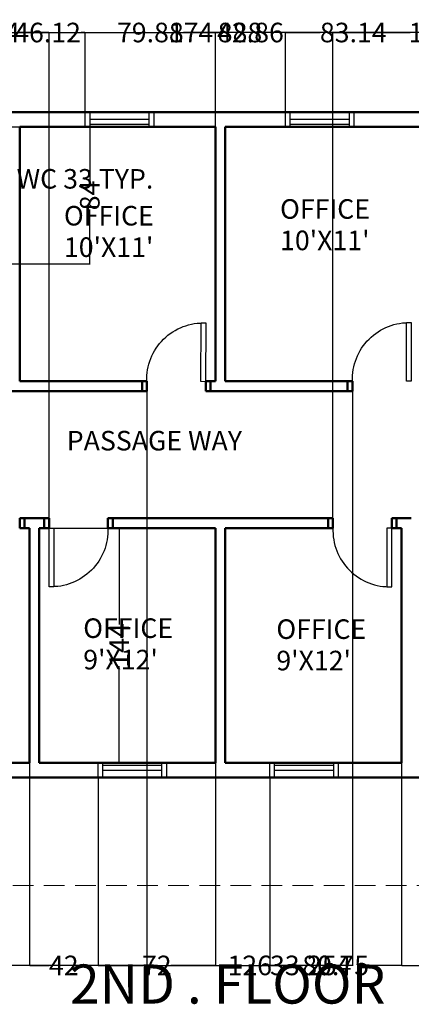
# Model space of a CAD drawing. Units: inches. Extents: x 128 to 1267, y -109 to 1208.
# Tile 7 of 8: x 546 to 786, y 592 to 1196. Entities that reach past the tile are written whole.
import ezdxf

# ---------------------------------------------------------------- set-up
doc = ezdxf.new("R2010")
doc.units = ezdxf.units.IN
doc.header["$MEASUREMENT"] = 0
doc.linetypes.add('DASHED', pattern=[19.05, 12.7, -6.35])
for name, color, linetype, lineweight in [('A-ANNO-DIMS', 2, 'Continuous', 18), ('A-ANNO-TEXT', 7, 'Continuous', 35), ('A-AREA-IDEN', 3, 'Continuous', 25), ('A-DOOR', 4, 'Continuous', 25), ('A-GLAZ', 3, 'Continuous', 25), ('A-ROOF-OVHD', 9, 'DASHED', 18), ('A-WALL', 7, 'Continuous', 50)]:
    doc.layers.add(name, color=color, linetype=linetype, lineweight=lineweight)
doc.styles.get("Standard").update_dxf_attribs({"font": 'arial.ttf'})
doc.dimstyles.get("Standard").update_dxf_attribs({"dimtxt": 12, "dimasz": 0.18, "dimexe": 0.18, "dimexo": 0.0625, "dimgap": 0.09, "dimtad": 0, "dimdec": 1, "dimzin": 0, "dimdsep": 46, "dimlunit": 3, "dimtxsty": 'Standard', "dimcen": 0.09, "dimadec": 0, "dimazin": 0, "dimtfac": 1, "dimtdec": 1, "dimtofl": 0, "dimtmove": 0, "dimatfit": 3, "dimfxl": 1, "dimtolj": 1, "dimtzin": 0, "dimarcsym": 0})

# ---------------------------------------------------------------- blocks, each defined once
blk = doc.blocks.new('DOOR-900')
blk.add_lwpolyline([(460.06, 187.64), (457.06, 187.64), (457.06, 151.64), (460.06, 151.64)], close=True)
blk.add_arc((458.56, 186.14), 34.53, 177.51045, 272.48955)
blk = doc.blocks.new('WIN-900')
for p, q in [((1102.06, 345.56), (1111.06, 345.56)), ((1102.06, 342.56), (1111.06, 342.56)), ((1103.56, 306.56), (1103.56, 342.56)), ((1106.56, 306.56), (1106.56, 342.56)), ((1111.06, 306.56), (1102.06, 306.56)), ((1111.06, 303.56), (1102.06, 303.56))]:
    blk.add_line(p, q)
blk = doc.blocks.new('*D16')
at = {"layer": 'A-ANNO-DIMS', "color": 0, "lineweight": -2, "transparency": 16777216}
for p, q in [((507.08, 1103.32), (507.08, 1098.25)), ((540.13, 1103.32), (540.13, 1098.25)), ((507.26, 1098.43), (539.95, 1098.43)), ((540.13, 1098.43), (540.31, 1098.43))]:
    blk.add_line(p, q, dxfattribs=at)
at = {"layer": 'A-ANNO-DIMS', "color": 0, "transparency": 16777216}
for points in [[(507.26, 1098.46), (507.26, 1098.4), (507.08, 1098.43)], [(539.95, 1098.46), (539.95, 1098.4), (540.13, 1098.43)]]:
    blk.add_solid(points, dxfattribs=at)
at = {"layer": 'Defpoints', "color": 0, "transparency": 16777216}
for p in [(507.08, 1103.38), (540.13, 1103.38), (540.13, 1098.43)]:
    blk.add_point(p, dxfattribs=at)
at = {"layer": 'A-ANNO-DIMS', "color": 0, "transparency": 16777216, "insert": (586.14, 1098.43), "char_height": 12, "attachment_point": 5}
blk.add_mtext('\\A1;WC 33 TYP.', dxfattribs=at)
blk = doc.blocks.new('*D93')
at = {"layer": 'A-ANNO-DIMS', "color": 0, "lineweight": -2, "transparency": 16777216}
for p, q in [((237.13, 664.93), (237.13, 1188.36)), ((237.31, 1188.18), (667.76, 1188.18)), ((1124.95, 1188.18), (694.49, 1188.18)), ((1125.13, 664.93), (1125.13, 1188.36))]:
    blk.add_line(p, q, dxfattribs=at)
at = {"layer": 'A-ANNO-DIMS', "color": 0, "transparency": 16777216}
for points in [[(237.31, 1188.21), (237.31, 1188.15), (237.13, 1188.18)], [(1124.95, 1188.21), (1124.95, 1188.15), (1125.13, 1188.18)]]:
    blk.add_solid(points, dxfattribs=at)
at = {"layer": 'Defpoints', "color": 0, "transparency": 16777216}
for p in [(1125.13, 1188.18), (237.13, 664.87), (1125.13, 664.87)]:
    blk.add_point(p, dxfattribs=at)
at = {"layer": 'A-ANNO-DIMS', "color": 0, "transparency": 16777216, "insert": (681.13, 1188.18), "char_height": 12, "attachment_point": 5}
blk.add_mtext('\\A1;888', dxfattribs=at)
blk = doc.blocks.new('*D103')
at = {"layer": 'A-ANNO-DIMS', "color": 0, "lineweight": -2, "transparency": 16777216}
for p, q in [((540.13, 1130.29), (540.13, 1188.36)), ((540.31, 1188.18), (542.67, 1188.18)), ((586.06, 1188.18), (583.7, 1188.18)), ((586.24, 1139.29), (586.24, 1188.36))]:
    blk.add_line(p, q, dxfattribs=at)
at = {"layer": 'A-ANNO-DIMS', "color": 0, "transparency": 16777216}
for points in [[(540.31, 1188.21), (540.31, 1188.15), (540.13, 1188.18)], [(586.06, 1188.21), (586.06, 1188.15), (586.24, 1188.18)]]:
    blk.add_solid(points, dxfattribs=at)
at = {"layer": 'Defpoints', "color": 0, "transparency": 16777216}
for p in [(586.24, 1188.18), (586.24, 1139.23), (540.13, 1130.23)]:
    blk.add_point(p, dxfattribs=at)
at = {"layer": 'A-ANNO-DIMS', "color": 0, "transparency": 16777216, "insert": (563.19, 1188.18), "char_height": 12, "attachment_point": 5}
blk.add_mtext('\\A1;46.12', dxfattribs=at)
blk = doc.blocks.new('*D104')
at = {"layer": 'A-ANNO-DIMS', "color": 0, "lineweight": -2, "transparency": 16777216}
for p, q in [((586.24, 1139.29), (586.24, 1188.36)), ((586.42, 1188.18), (605.89, 1188.18)), ((665.95, 1188.18), (646.49, 1188.18)), ((666.13, 1130.29), (666.13, 1188.36))]:
    blk.add_line(p, q, dxfattribs=at)
at = {"layer": 'A-ANNO-DIMS', "color": 0, "transparency": 16777216}
for points in [[(586.42, 1188.21), (586.42, 1188.15), (586.24, 1188.18)], [(665.95, 1188.21), (665.95, 1188.15), (666.13, 1188.18)]]:
    blk.add_solid(points, dxfattribs=at)
at = {"layer": 'Defpoints', "color": 0, "transparency": 16777216}
for p in [(666.13, 1188.18), (586.24, 1139.23), (666.13, 1130.23)]:
    blk.add_point(p, dxfattribs=at)
at = {"layer": 'A-ANNO-DIMS', "color": 0, "transparency": 16777216, "insert": (626.19, 1188.18), "char_height": 12, "attachment_point": 5}
blk.add_mtext('\\A1;79.88', dxfattribs=at)
blk = doc.blocks.new('*D105')
at = {"layer": 'A-ANNO-DIMS', "color": 0, "lineweight": -2, "transparency": 16777216}
for p, q in [((666.13, 1130.29), (666.13, 1188.36)), ((666.31, 1188.18), (666.98, 1188.18)), ((708.81, 1188.18), (708.13, 1188.18)), ((708.99, 1139.29), (708.99, 1188.36))]:
    blk.add_line(p, q, dxfattribs=at)
at = {"layer": 'A-ANNO-DIMS', "color": 0, "transparency": 16777216}
for points in [[(666.31, 1188.21), (666.31, 1188.15), (666.13, 1188.18)], [(708.81, 1188.21), (708.81, 1188.15), (708.99, 1188.18)]]:
    blk.add_solid(points, dxfattribs=at)
at = {"layer": 'Defpoints', "color": 0, "transparency": 16777216}
for p in [(708.99, 1188.18), (708.99, 1139.23), (666.13, 1130.23)]:
    blk.add_point(p, dxfattribs=at)
at = {"layer": 'A-ANNO-DIMS', "color": 0, "transparency": 16777216, "insert": (687.56, 1188.18), "char_height": 12, "attachment_point": 5}
blk.add_mtext('\\A1;42.86', dxfattribs=at)
blk = doc.blocks.new('*D106')
at = {"layer": 'A-ANNO-DIMS', "color": 0, "lineweight": -2, "transparency": 16777216}
for p, q in [((708.99, 1139.29), (708.99, 1188.36)), ((709.17, 1188.18), (730.24, 1188.18)), ((791.95, 1188.18), (770.88, 1188.18)), ((792.13, 1130.29), (792.13, 1188.36))]:
    blk.add_line(p, q, dxfattribs=at)
at = {"layer": 'A-ANNO-DIMS', "color": 0, "transparency": 16777216}
for points in [[(709.17, 1188.21), (709.17, 1188.15), (708.99, 1188.18)], [(791.95, 1188.21), (791.95, 1188.15), (792.13, 1188.18)]]:
    blk.add_solid(points, dxfattribs=at)
at = {"layer": 'Defpoints', "color": 0, "transparency": 16777216}
for p in [(792.13, 1188.18), (708.99, 1139.23), (792.13, 1130.23)]:
    blk.add_point(p, dxfattribs=at)
at = {"layer": 'A-ANNO-DIMS', "color": 0, "transparency": 16777216, "insert": (750.56, 1188.18), "char_height": 12, "attachment_point": 5}
blk.add_mtext('\\A1;83.14', dxfattribs=at)
blk = doc.blocks.new('*D115')
at = {"layer": 'A-ANNO-DIMS', "color": 0, "lineweight": -2, "transparency": 16777216}
for p, q in [((552.13, 740.16), (552.13, 615.74)), ((455.08, 731.16), (455.08, 615.74)), ((455.26, 615.92), (483.22, 615.92)), ((551.95, 615.92), (523.98, 615.92))]:
    blk.add_line(p, q, dxfattribs=at)
at = {"layer": 'A-ANNO-DIMS', "color": 0, "transparency": 16777216}
for points in [[(455.26, 615.95), (455.26, 615.89), (455.08, 615.92)], [(551.95, 615.95), (551.95, 615.89), (552.13, 615.92)]]:
    blk.add_solid(points, dxfattribs=at)
at = {"layer": 'Defpoints', "color": 0, "transparency": 16777216}
for p in [(552.13, 740.23), (455.08, 731.23), (552.13, 615.92)]:
    blk.add_point(p, dxfattribs=at)
at = {"layer": 'A-ANNO-DIMS', "color": 0, "transparency": 16777216, "insert": (503.6, 615.92), "char_height": 12, "attachment_point": 5}
blk.add_mtext('\\A1;97.05', dxfattribs=at)
blk = doc.blocks.new('*D116')
at = {"layer": 'A-ANNO-DIMS', "color": 0, "lineweight": -2, "transparency": 16777216}
for p, q in [((552.13, 740.16), (552.13, 615.74)), ((594.13, 731.16), (594.13, 615.74)), ((552.31, 615.92), (564.26, 615.92)), ((593.95, 615.92), (581.99, 615.92))]:
    blk.add_line(p, q, dxfattribs=at)
at = {"layer": 'A-ANNO-DIMS', "color": 0, "transparency": 16777216}
for points in [[(552.31, 615.95), (552.31, 615.89), (552.13, 615.92)], [(593.95, 615.95), (593.95, 615.89), (594.13, 615.92)]]:
    blk.add_solid(points, dxfattribs=at)
at = {"layer": 'Defpoints', "color": 0, "transparency": 16777216}
for p in [(552.13, 740.23), (594.13, 731.23), (594.13, 615.92)]:
    blk.add_point(p, dxfattribs=at)
at = {"layer": 'A-ANNO-DIMS', "color": 0, "transparency": 16777216, "insert": (573.13, 615.92), "char_height": 12, "attachment_point": 5}
blk.add_mtext('\\A1;42', dxfattribs=at)
blk = doc.blocks.new('*D117')
at = {"layer": 'A-ANNO-DIMS', "color": 0, "lineweight": -2, "transparency": 16777216}
for p, q in [((666.13, 740.16), (666.13, 615.74)), ((594.13, 731.16), (594.13, 615.74)), ((594.31, 615.92), (621.55, 615.92)), ((665.95, 615.92), (638.7, 615.92))]:
    blk.add_line(p, q, dxfattribs=at)
at = {"layer": 'A-ANNO-DIMS', "color": 0, "transparency": 16777216}
for points in [[(594.31, 615.95), (594.31, 615.89), (594.13, 615.92)], [(665.95, 615.95), (665.95, 615.89), (666.13, 615.92)]]:
    blk.add_solid(points, dxfattribs=at)
at = {"layer": 'Defpoints', "color": 0, "transparency": 16777216}
for p in [(666.13, 740.23), (594.13, 731.23), (666.13, 615.92)]:
    blk.add_point(p, dxfattribs=at)
at = {"layer": 'A-ANNO-DIMS', "color": 0, "transparency": 16777216, "insert": (630.13, 615.92), "char_height": 12, "attachment_point": 5}
blk.add_mtext('\\A1;72', dxfattribs=at)
blk = doc.blocks.new('*D118')
at = {"layer": 'A-ANNO-DIMS', "color": 0, "lineweight": -2, "transparency": 16777216}
for p, q in [((666.13, 740.16), (666.13, 615.74)), ((699.38, 731.16), (699.38, 615.74)), ((666.31, 615.92), (699.2, 615.92)), ((699.38, 615.92), (699.56, 615.92))]:
    blk.add_line(p, q, dxfattribs=at)
at = {"layer": 'A-ANNO-DIMS', "color": 0, "transparency": 16777216}
for points in [[(666.31, 615.95), (666.31, 615.89), (666.13, 615.92)], [(699.2, 615.95), (699.2, 615.89), (699.38, 615.92)]]:
    blk.add_solid(points, dxfattribs=at)
at = {"layer": 'Defpoints', "color": 0, "transparency": 16777216}
for p in [(666.13, 740.23), (699.38, 731.23), (699.38, 615.92)]:
    blk.add_point(p, dxfattribs=at)
at = {"layer": 'A-ANNO-DIMS', "color": 0, "transparency": 16777216, "insert": (724.53, 615.92), "char_height": 12, "attachment_point": 5}
blk.add_mtext('\\A1;33.254', dxfattribs=at)
blk = doc.blocks.new('*D119')
at = {"layer": 'A-ANNO-DIMS', "color": 0, "lineweight": -2, "transparency": 16777216}
for p, q in [((780.13, 740.16), (780.13, 615.74)), ((699.38, 731.16), (699.38, 615.74)), ((699.56, 615.92), (719.36, 615.92)), ((779.95, 615.92), (760.14, 615.92))]:
    blk.add_line(p, q, dxfattribs=at)
at = {"layer": 'A-ANNO-DIMS', "color": 0, "transparency": 16777216}
for points in [[(699.56, 615.95), (699.56, 615.89), (699.38, 615.92)], [(779.95, 615.95), (779.95, 615.89), (780.13, 615.92)]]:
    blk.add_solid(points, dxfattribs=at)
at = {"layer": 'Defpoints', "color": 0, "transparency": 16777216}
for p in [(780.13, 740.23), (699.38, 731.23), (780.13, 615.92)]:
    blk.add_point(p, dxfattribs=at)
at = {"layer": 'A-ANNO-DIMS', "color": 0, "transparency": 16777216, "insert": (739.75, 615.92), "char_height": 12, "attachment_point": 5}
blk.add_mtext('\\A1;80.75', dxfattribs=at)
blk = doc.blocks.new('*D120')
at = {"layer": 'A-ANNO-DIMS', "color": 0, "lineweight": -2, "transparency": 16777216}
for p, q in [((780.13, 740.16), (780.13, 615.74)), ((802.84, 731.16), (802.84, 615.74)), ((780.31, 615.92), (802.66, 615.92)), ((802.84, 615.92), (803.02, 615.92))]:
    blk.add_line(p, q, dxfattribs=at)
at = {"layer": 'A-ANNO-DIMS', "color": 0, "transparency": 16777216}
for points in [[(780.31, 615.95), (780.31, 615.89), (780.13, 615.92)], [(802.66, 615.95), (802.66, 615.89), (802.84, 615.92)]]:
    blk.add_solid(points, dxfattribs=at)
at = {"layer": 'Defpoints', "color": 0, "transparency": 16777216}
for p in [(780.13, 740.23), (802.84, 731.23), (802.84, 615.92)]:
    blk.add_point(p, dxfattribs=at)
at = {"layer": 'A-ANNO-DIMS', "color": 0, "transparency": 16777216, "insert": (828.1, 615.92), "char_height": 12, "attachment_point": 5}
blk.add_mtext('\\A1;22.714', dxfattribs=at)
blk = doc.blocks.new('*D135')
at = {"layer": 'A-ANNO-DIMS', "color": 0, "lineweight": -2, "transparency": 16777216}
for p, q in [((540.19, 1130.23), (589.26, 1130.23)), ((589.08, 1130.05), (589.08, 1096.89)), ((589.08, 1046.41), (589.08, 1079.56)), ((540.19, 1046.23), (589.26, 1046.23))]:
    blk.add_line(p, q, dxfattribs=at)
at = {"layer": 'A-ANNO-DIMS', "color": 0, "transparency": 16777216}
for points in [[(589.05, 1130.05), (589.11, 1130.05), (589.08, 1130.23)], [(589.05, 1046.41), (589.11, 1046.41), (589.08, 1046.23)]]:
    blk.add_solid(points, dxfattribs=at)
at = {"layer": 'Defpoints', "color": 0, "transparency": 16777216}
for p in [(540.13, 1130.23), (540.13, 1046.23), (589.08, 1046.23)]:
    blk.add_point(p, dxfattribs=at)
at = {"layer": 'A-ANNO-DIMS', "color": 0, "transparency": 16777216, "insert": (589.08, 1088.23), "char_height": 12, "attachment_point": 5, "rotation": 90}
blk.add_mtext('\\A1;84', dxfattribs=at)
blk = doc.blocks.new('*D139')
at = {"layer": 'A-ANNO-DIMS', "color": 0, "lineweight": -2, "transparency": 16777216}
for p, q in [((558.19, 884.23), (607.26, 884.23)), ((607.08, 884.05), (607.08, 824.98)), ((607.08, 740.41), (607.08, 799.47)), ((558.19, 740.23), (607.26, 740.23))]:
    blk.add_line(p, q, dxfattribs=at)
at = {"layer": 'A-ANNO-DIMS', "color": 0, "transparency": 16777216}
for points in [[(607.05, 884.05), (607.11, 884.05), (607.08, 884.23)], [(607.05, 740.41), (607.11, 740.41), (607.08, 740.23)]]:
    blk.add_solid(points, dxfattribs=at)
at = {"layer": 'Defpoints', "color": 0, "transparency": 16777216}
for p in [(558.13, 884.23), (558.13, 740.23), (607.08, 740.23)]:
    blk.add_point(p, dxfattribs=at)
at = {"layer": 'A-ANNO-DIMS', "color": 0, "transparency": 16777216, "insert": (607.08, 812.23), "char_height": 12, "attachment_point": 5, "rotation": 90}
blk.add_mtext('\\A1;144', dxfattribs=at)
blk = doc.blocks.new('*D148')
at = {"layer": 'A-ANNO-DIMS', "color": 0, "lineweight": -2, "transparency": 16777216}
for p, q in [((420.13, 968.16), (420.13, 615.74)), ((624.13, 968.16), (624.13, 615.74)), ((420.31, 615.92), (508.7, 615.92)), ((623.95, 615.92), (535.55, 615.92))]:
    blk.add_line(p, q, dxfattribs=at)
at = {"layer": 'A-ANNO-DIMS', "color": 0, "transparency": 16777216}
for points in [[(420.31, 615.95), (420.31, 615.89), (420.13, 615.92)], [(623.95, 615.95), (623.95, 615.89), (624.13, 615.92)]]:
    blk.add_solid(points, dxfattribs=at)
at = {"layer": 'Defpoints', "color": 0, "transparency": 16777216}
for p in [(420.13, 968.23), (624.13, 968.23), (624.13, 615.92)]:
    blk.add_point(p, dxfattribs=at)
at = {"layer": 'A-ANNO-DIMS', "color": 0, "transparency": 16777216, "insert": (522.13, 615.92), "char_height": 12, "attachment_point": 5}
blk.add_mtext('\\A1;204', dxfattribs=at)
blk = doc.blocks.new('*D149')
at = {"layer": 'A-ANNO-DIMS', "color": 0, "lineweight": -2, "transparency": 16777216}
for p, q in [((624.13, 968.16), (624.13, 615.74)), ((750.13, 968.16), (750.13, 615.74)), ((624.31, 615.92), (674.35, 615.92)), ((749.95, 615.92), (699.9, 615.92))]:
    blk.add_line(p, q, dxfattribs=at)
at = {"layer": 'A-ANNO-DIMS', "color": 0, "transparency": 16777216}
for points in [[(624.31, 615.95), (624.31, 615.89), (624.13, 615.92)], [(749.95, 615.95), (749.95, 615.89), (750.13, 615.92)]]:
    blk.add_solid(points, dxfattribs=at)
at = {"layer": 'Defpoints', "color": 0, "transparency": 16777216}
for p in [(624.13, 968.23), (750.13, 968.23), (750.13, 615.92)]:
    blk.add_point(p, dxfattribs=at)
at = {"layer": 'A-ANNO-DIMS', "color": 0, "transparency": 16777216, "insert": (687.13, 615.92), "char_height": 12, "attachment_point": 5}
blk.add_mtext('\\A1;126', dxfattribs=at)
blk = doc.blocks.new('*D153')
at = {"layer": 'A-ANNO-DIMS', "color": 0, "lineweight": -2, "transparency": 16777216}
for p, q in [((510.13, 890.29), (510.13, 1188.36)), ((510.31, 1188.18), (528.47, 1188.18)), ((563.95, 1188.18), (545.79, 1188.18)), ((564.13, 890.29), (564.13, 1188.36))]:
    blk.add_line(p, q, dxfattribs=at)
at = {"layer": 'A-ANNO-DIMS', "color": 0, "transparency": 16777216}
for points in [[(510.31, 1188.21), (510.31, 1188.15), (510.13, 1188.18)], [(563.95, 1188.21), (563.95, 1188.15), (564.13, 1188.18)]]:
    blk.add_solid(points, dxfattribs=at)
at = {"layer": 'Defpoints', "color": 0, "transparency": 16777216}
for p in [(564.13, 1188.18), (510.13, 890.23), (564.13, 890.23)]:
    blk.add_point(p, dxfattribs=at)
at = {"layer": 'A-ANNO-DIMS', "color": 0, "transparency": 16777216, "insert": (537.13, 1188.18), "char_height": 12, "attachment_point": 5}
blk.add_mtext('\\A1;54', dxfattribs=at)
blk = doc.blocks.new('*D154')
at = {"layer": 'A-ANNO-DIMS', "color": 0, "lineweight": -2, "transparency": 16777216}
for p, q in [((564.13, 890.29), (564.13, 1188.36)), ((564.31, 1188.18), (638.37, 1188.18)), ((737.95, 1188.18), (663.88, 1188.18)), ((738.13, 890.29), (738.13, 1188.36))]:
    blk.add_line(p, q, dxfattribs=at)
at = {"layer": 'A-ANNO-DIMS', "color": 0, "transparency": 16777216}
for points in [[(564.31, 1188.21), (564.31, 1188.15), (564.13, 1188.18)], [(737.95, 1188.21), (737.95, 1188.15), (738.13, 1188.18)]]:
    blk.add_solid(points, dxfattribs=at)
at = {"layer": 'Defpoints', "color": 0, "transparency": 16777216}
for p in [(738.13, 1188.18), (564.13, 890.23), (738.13, 890.23)]:
    blk.add_point(p, dxfattribs=at)
at = {"layer": 'A-ANNO-DIMS', "color": 0, "transparency": 16777216, "insert": (651.13, 1188.18), "char_height": 12, "attachment_point": 5}
blk.add_mtext('\\A1;174', dxfattribs=at)
blk = doc.blocks.new('*D155')
at = {"layer": 'A-ANNO-DIMS', "color": 0, "lineweight": -2, "transparency": 16777216}
for p, q in [((738.13, 890.29), (738.13, 1188.36)), ((738.31, 1188.18), (785.37, 1188.18)), ((857.95, 1188.18), (810.89, 1188.18)), ((858.13, 890.29), (858.13, 1188.36))]:
    blk.add_line(p, q, dxfattribs=at)
at = {"layer": 'A-ANNO-DIMS', "color": 0, "transparency": 16777216}
for points in [[(738.31, 1188.21), (738.31, 1188.15), (738.13, 1188.18)], [(857.95, 1188.21), (857.95, 1188.15), (858.13, 1188.18)]]:
    blk.add_solid(points, dxfattribs=at)
at = {"layer": 'Defpoints', "color": 0, "transparency": 16777216}
for p in [(858.13, 1188.18), (738.13, 890.23), (858.13, 890.23)]:
    blk.add_point(p, dxfattribs=at)
at = {"layer": 'A-ANNO-DIMS', "color": 0, "transparency": 16777216, "insert": (798.13, 1188.18), "char_height": 12, "attachment_point": 5}
blk.add_mtext('\\A1;120', dxfattribs=at)

msp = doc.modelspace()

# ---------------------------------------------------------------- linework, layer by layer
at = {"layer": 'A-ROOF-OVHD'}
msp.add_line((237.1268, 664.8687), (1125.1268, 664.8687), dxfattribs=at)
at = {"layer": 'A-WALL'}
for p, q in [((546.1268, 974.2265), (546.1268, 1130.2265)), ((666.1268, 1130.2265), (546.1268, 1130.2265)), ((666.1268, 974.2265), (666.1268, 1130.2265)), ((672.1268, 974.2265), (672.1268, 1130.2265)), ((792.1268, 1130.2265), (672.1268, 1130.2265)), ((624.1268, 974.2265), (546.1268, 974.2265)), ((621.1268, 974.2265), (621.1268, 968.2265)), ((624.1268, 974.2265), (624.1268, 968.2265)), ((666.1268, 974.2265), (660.1268, 974.2265)), ((660.1268, 974.2265), (660.1268, 968.2265)), ((663.1268, 974.2265), (663.1268, 968.2265)), ((750.1268, 974.2265), (672.1268, 974.2265)), ((747.1268, 974.2265), (747.1268, 968.2265)), ((750.1268, 974.2265), (750.1268, 968.2265)), ((624.1268, 968.2265), (540.1268, 968.2265)), ((750.1268, 968.2265), (660.1268, 968.2265)), ((546.1268, 884.2265), (546.1268, 890.2265)), ((546.1268, 890.2265), (564.1268, 890.2265)), ((549.1268, 884.2265), (549.1268, 890.2265)), ((561.1268, 884.2265), (561.1268, 890.2265)), ((564.1268, 884.2265), (564.1268, 890.2265)), ((600.1268, 884.2265), (600.1268, 890.2265)), ((600.1268, 890.2265), (738.1268, 890.2265)), ((603.1268, 884.2265), (603.1268, 890.2265)), ((735.1268, 884.2265), (735.1268, 890.2265)), ((738.1268, 884.2265), (738.1268, 890.2265)), ((774.1268, 884.2265), (774.1268, 890.2265)), ((774.1268, 890.2265), (786.1268, 890.2265)), ((777.1268, 884.2265), (777.1268, 890.2265)), ((546.1268, 884.2265), (552.1268, 884.2265)), ((552.1268, 884.2265), (552.1268, 740.2265)), ((558.1268, 884.2265), (558.1268, 740.2265)), ((558.1268, 884.2265), (564.1268, 884.2265)), ((600.1268, 884.2265), (666.1268, 884.2265)), ((666.1268, 884.2265), (666.1268, 740.2265)), ((672.1268, 884.2265), (672.1268, 740.2265)), ((672.1268, 884.2265), (738.1268, 884.2265)), ((774.1268, 884.2265), (780.1268, 884.2265)), ((780.1268, 884.2265), (780.1268, 740.2265)), ((246.1268, 740.2265), (552.1268, 740.2265)), ((444.1268, 740.2265), (552.1268, 740.2265)), ((444.1268, 740.2265), (552.1268, 740.2265)), ((558.1268, 740.2265), (594.1268, 740.2265)), ((558.1268, 740.2265), (666.1268, 740.2265)), ((672.1268, 740.2265), (780.1268, 740.2265))]:
    msp.add_line(p, q, dxfattribs=at)
msp.add_lwpolyline([(1110.1268, 731.2265), (1125.1268, 731.2265), (1125.1268, 1139.2265), (237.1268, 1139.2265), (237.1268, 731.2265), (1038.1268, 731.2265)], dxfattribs=at)

# ---------------------------------------------------------------- block references
at = {"layer": 'A-DOOR', "extrusion": (0, 0, -1), "zscale": -1}
for p, rotation in [((-201.0289, 1164.1499), 180.3133457630147), ((-326.0707, 1161.8664), 180)]:
    msp.add_blockref('DOOR-900', p, dxfattribs=dict(at, rotation=rotation))
msp.add_blockref('DOOR-900', (-1024.1828, 696.5866), dxfattribs=at)
at = {"layer": 'A-DOOR'}
msp.add_blockref('DOOR-900', (314.0707, 696.5866), dxfattribs=at)
at = {"layer": 'A-GLAZ'}
for p, rotation in [((931.8065, 28.1705), 90.00000000000095), ((1054.5475, 28.1705), 90.0000000000011), ((290.5645, 1842.2825), 270.0000000000002), ((395.818, 1842.2825), 270.0000000000003)]:
    msp.add_blockref('WIN-900', p, dxfattribs=dict(at, rotation=rotation))

# ---------------------------------------------------------------- texts
at = {"layer": 'A-ANNO-TEXT'}
msp.add_text('2ND . FLOOR', height=24, dxfattribs=at).set_placement((576.914, 592.4923))
at = {"layer": 'A-AREA-IDEN'}
for s, p in [('OFFICE', (573.2286, 1069.7979)), ('OFFICE', (705.6979, 1073.9433)), ("10'X11'", (573.2286, 1050.5209)), ("10'X11'", (705.6979, 1054.6663)), ('PASSAGE WAY', (574.9737, 931.8027)), ('OFFICE', (585.0521, 816.7941)), ('OFFICE', (703.4201, 816.2028)), ("9'X12'", (585.0521, 797.5172)), ("9'X12'", (703.4201, 796.9258))]:
    msp.add_text(s, height=12, dxfattribs=at).set_placement(p)

# ---------------------------------------------------------------- dimensions: what is measured, and where the dimension line sits
at = {"layer": 'A-ANNO-DIMS'}
for base, p1, p2, override, picture, middle in [((1125.1268, 1188.1765), (237.1268, 664.8687), (1125.1268, 664.8687), {"dimdec": 0, "dimlfac": 1, "dimrnd": 0, "dimzin": 0, "dimdsep": 46, "dimlunit": 2}, '*D93', (681.1268, 1188.1765)), ((564.1268, 1188.1765), (510.1268, 890.2265), (564.1268, 890.2265), {"dimdec": 0, "dimlfac": 1, "dimrnd": 0, "dimzin": 0, "dimdsep": 46, "dimlunit": 2}, '*D153', (537.1268, 1188.1765)), ((586.2442, 1188.1765), (540.1268, 1130.2265), (586.2442, 1139.2265), {"dimdec": 2, "dimlfac": 1, "dimrnd": 0, "dimzin": 0, "dimdsep": 46, "dimlunit": 2}, '*D103', (563.1855, 1188.1765)), ((738.1268, 1188.1765), (564.1268, 890.2265), (738.1268, 890.2265), {"dimdec": 0, "dimlfac": 1, "dimrnd": 0, "dimzin": 0, "dimdsep": 46, "dimlunit": 2}, '*D154', (651.1268, 1188.1765)), ((666.1268, 1188.1765), (586.2442, 1139.2265), (666.1268, 1130.2265), {"dimdec": 2, "dimlfac": 1, "dimrnd": 0, "dimzin": 0, "dimdsep": 46, "dimlunit": 2}, '*D104', (626.1855, 1188.1765)), ((708.9852, 1188.1765), (666.1268, 1130.2265), (708.9852, 1139.2265), {"dimdec": 2, "dimlfac": 1, "dimrnd": 0, "dimzin": 0, "dimdsep": 46, "dimlunit": 2}, '*D105', (687.556, 1188.1765)), ((792.1268, 1188.1765), (708.9852, 1139.2265), (792.1268, 1130.2265), {"dimdec": 2, "dimlfac": 1, "dimrnd": 0, "dimzin": 0, "dimdsep": 46, "dimlunit": 2}, '*D106', (750.556, 1188.1765)), ((858.1268, 1188.1765), (738.1268, 890.2265), (858.1268, 890.2265), {"dimdec": 0, "dimlfac": 1, "dimrnd": 0, "dimzin": 0, "dimdsep": 46, "dimlunit": 2}, '*D155', (798.1268, 1188.1765)), ((624.1268, 615.9187), (420.1268, 968.2265), (624.1268, 968.2265), {"dimdec": 0, "dimlfac": 1, "dimrnd": 0, "dimzin": 0, "dimdsep": 46, "dimlunit": 2}, '*D148', (522.1268, 615.9187)), ((750.1268, 615.9187), (624.1268, 968.2265), (750.1268, 968.2265), {"dimdec": 0, "dimlfac": 1, "dimrnd": 0, "dimzin": 0, "dimdsep": 46, "dimlunit": 2}, '*D149', (687.1268, 615.9187)), ((552.1268, 615.9187), (455.0763, 731.2265), (552.1268, 740.2265), {"dimdec": 2, "dimlfac": 1, "dimrnd": 0, "dimzin": 0, "dimdsep": 46, "dimlunit": 2}, '*D115', (503.6015, 615.9187)), ((594.1268, 615.9187), (552.1268, 740.2265), (594.1268, 731.2265), {"dimdec": 0, "dimlfac": 1, "dimrnd": 0, "dimzin": 0, "dimdsep": 46, "dimlunit": 2}, '*D116', (573.1268, 615.9187)), ((666.1268, 615.9187), (594.1268, 731.2265), (666.1268, 740.2265), {"dimdec": 0, "dimlfac": 1, "dimrnd": 0, "dimzin": 0, "dimdsep": 46, "dimlunit": 2}, '*D117', (630.1268, 615.9187)), ((699.3804, 615.9187), (666.1268, 740.2265), (699.3804, 731.2265), {"dimdec": 3, "dimlfac": 1, "dimrnd": 0, "dimzin": 0, "dimdsep": 46, "dimlunit": 2}, '*D118', (724.5303, 615.9187)), ((780.1268, 615.9187), (699.3804, 731.2265), (780.1268, 740.2265), {"dimdec": 2, "dimlfac": 1, "dimrnd": 0, "dimzin": 0, "dimdsep": 46, "dimlunit": 2}, '*D119', (739.7536, 615.9187)), ((802.8411, 615.9187), (780.1268, 740.2265), (802.8411, 731.2265), {"dimdec": 3, "dimlfac": 1, "dimrnd": 0, "dimzin": 0, "dimdsep": 46, "dimlunit": 2}, '*D120', (828.0975, 615.9187))]:
    dim = msp.add_linear_dim(base=base, p1=p1, p2=p2, dimstyle='Standard', override=override, dxfattribs=at)
    dim.commit()
    dim.dimension.update_dxf_attribs({"geometry": picture, "text_midpoint": middle})
for base, p1, p2, picture, middle in [((589.0768, 1046.2265), (540.1268, 1130.2265), (540.1268, 1046.2265), '*D135', (589.0768, 1088.2265)), ((607.0768, 740.2265), (558.1268, 884.2265), (558.1268, 740.2265), '*D139', (607.0768, 812.2265))]:
    dim = msp.add_linear_dim(base=base, p1=p1, p2=p2, angle=270, dimstyle='Standard', override={"dimdec": 0, "dimlfac": 1, "dimrnd": 0, "dimzin": 0, "dimdsep": 46, "dimlunit": 2}, dxfattribs=at)
    dim.commit()
    dim.dimension.update_dxf_attribs({"geometry": picture, "text_midpoint": middle})
dim = msp.add_linear_dim(base=(540.1268, 1098.426), p1=(507.0805, 1103.3829), p2=(540.1268, 1103.3829), text='WC <> TYP.', dimstyle='Standard', override={"dimdec": 0, "dimrnd": 0, "dimzin": 0, "dimlunit": 2}, dxfattribs=at)
dim.commit()
dim.dimension.update_dxf_attribs({"geometry": '*D16', "text_midpoint": (586.1416, 1098.426)})

doc.saveas('drawing.dxf')
